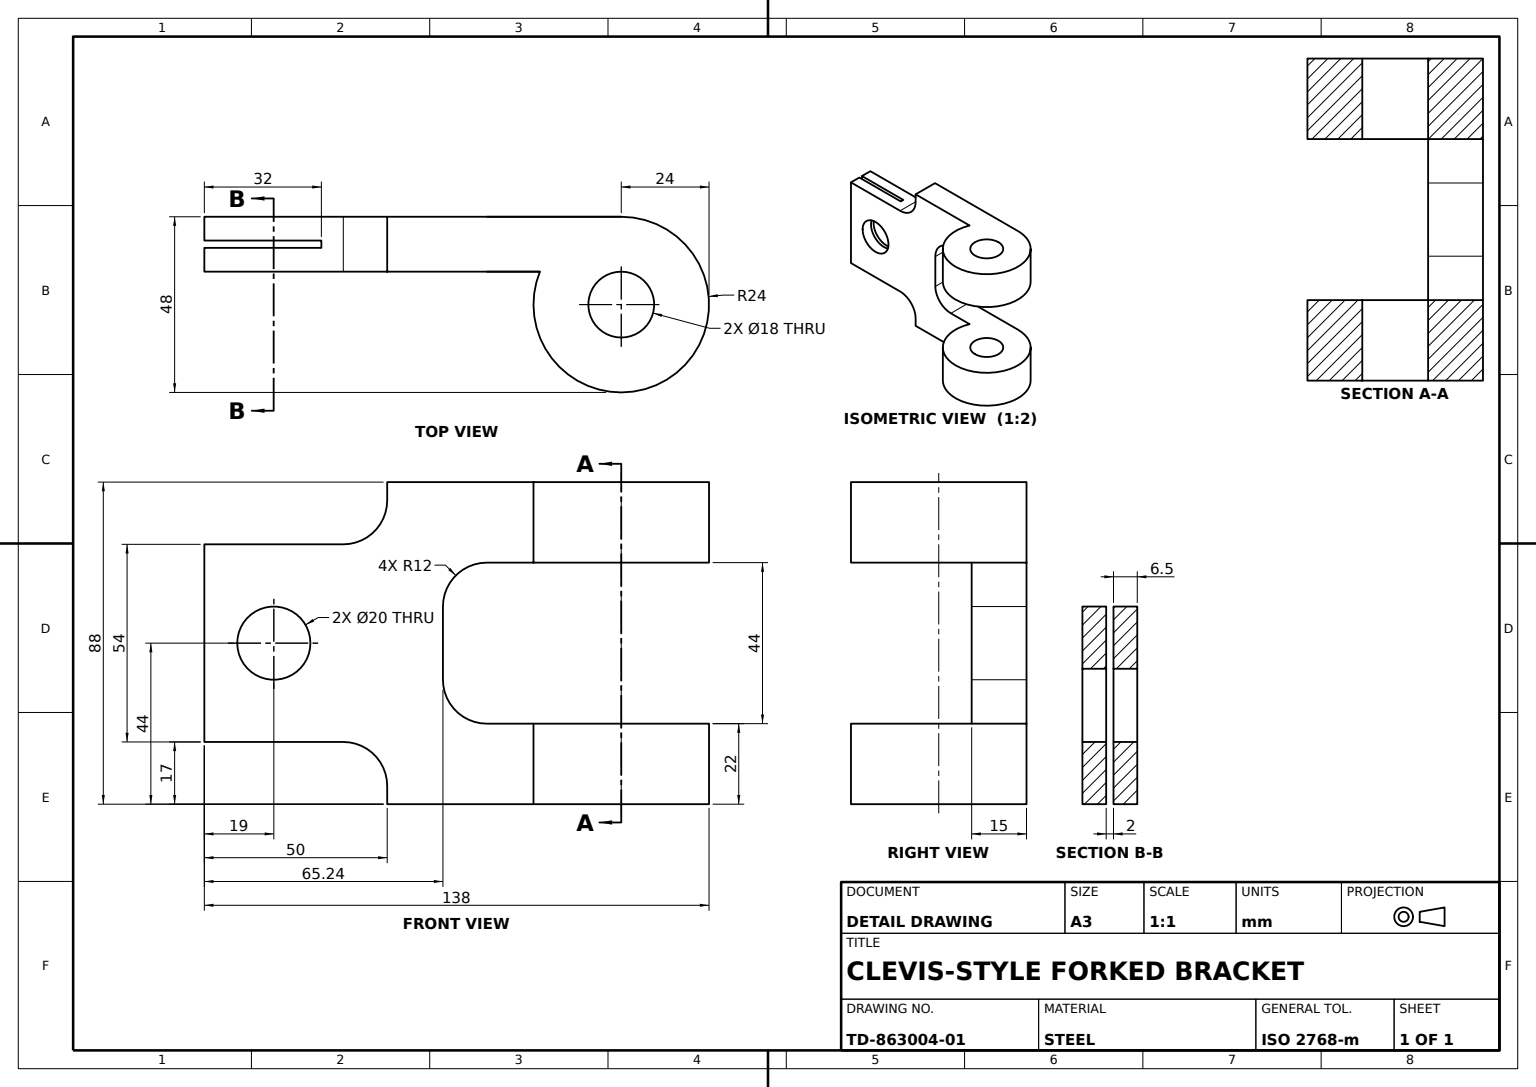
SolidWorks part; units mm, degrees
material "Plain Carbon Steel"
ref_plane "Front Plane" through (0, 0, 0) normal (0, 0, 1) x (1, 0, 0)
ref_plane "Top Plane" through (0, 0, 0) normal (0, 1, 0) x (1, 0, 0)
ref_plane "Right Plane" through (0, 0, 0) normal (1, 0, 0) x (0, 0, -1)
sketch "Base Plate Profile" plane through (0, 0, 0) normal (0, 0, 1) x (1, 0, 0)
  line L0 (0, 0) -> (64, 0)
  line L1 (0, 0) -> (0, -88)
  line L2 (0, -88) -> (64, -88)
  line L3 (64, -88) -> (64, -66)
  line L4 (64, -66) -> (27.24, -66)
  line L5 (15.24, -54) -> (15.24, -34)
  line L6 (27.24, -22) -> (64, -22)
  line L7 (64, -22) -> (64, 0)
  arc A0 (15.24, -54) -> (27.24, -66) centre (27.24, -54) ccw
  arc A1 (27.24, -22) -> (15.24, -34) centre (27.24, -34) ccw
  dimension "D1" = 12
  dimension "D3" = 12
  dimension "D2" = 22
  dimension "D4" = 44
  dimension "D5" = 64
  dimension "D6" = 88
  dimension "D7" = 66
  dimension "D8" = 36.76
extrude "Base Plate" add sketch "Base Plate Profile" along normal blind 15
sketch "Pivot Boss 1 Profile" plane through (0, 0, 0) normal (0, 1, 0) x (1, 0, 0)
  line L0 (0, -15) -> (0, 0) construction
  line L1 (64, 0) -> (0, 0) construction
  circle A0 centre (64, -24) radius 24
  dimension "D1" = 48
  dimension "D2" = 64
  dimension "D3" = 24
extrude "Pivot Boss 1" add sketch "Pivot Boss 1 Profile" against normal blind 22
sketch "Pivot Boss 2 Profile" plane through (0, -88, 0) normal (0, -1, 0) x (1, 0, 0)
  circle A0 centre (64, 24) radius 24
  dimension "D1" = 48
extrude "Pivot Boss 2" add sketch "Pivot Boss 2 Profile" against normal blind 22
sketch "Upright Web Profile" plane through (0, 0, 0) normal (0, 0, -1) x (-1, 0, 0)
  line L0 (0, -44) -> (0, -17)
  line L1 (0, 0) -> (0, -88) construction
  line L2 (0, -44) -> (0, -71)
  line L3 (12, -71) -> (50, -71)
  line L4 (50, -71) -> (50, -17)
  line L5 (50, -17) -> (12, -17)
  line L6 (0, -83) -> (0, -71)
  line L7 (0, -5) -> (0, -17)
  line L8 (-64, 0) -> (0, 0) construction
  arc A0 (0, -5) -> (12, -17) centre (12, -5) ccw
  arc A1 (12, -71) -> (0, -83) centre (12, -83) ccw
  dimension "D1" = 12
  dimension "D2" = 50
  dimension "D3" = 17
extrude "Upright Web" add sketch "Upright Web Profile" against normal blind 15
sketch "Web Slot Profile" plane through (0, -17, 0) normal (0, 1, 0) x (1, 0, 0)
  line L0 (-50, -7.5) -> (-50, -6.5)
  line L1 (-50, -15) -> (-50, 0) construction
  line L2 (-50, -6.5) -> (-18, -6.5)
  line L3 (-18, -6.5) -> (-18, -8.5)
  line L4 (-18, -8.5) -> (-50, -8.5)
  line L5 (-50, -8.5) -> (-50, -7.5)
  line L6 (-50, 0) -> (-12, 0) construction
  dimension "D1" = 32
  dimension "D2" = 6.5
extrude "Web Slot" cut sketch "Web Slot Profile" against normal blind 55
sketch "Web Hole Profile" plane through (0, 0, 15) normal (0, 0, 1) x (1, 0, 0)
  line L0 (41.7514, 0) -> (41.7514, -22) construction
  line L1 (41.7514, 0) -> (0, 0) construction
  circle A0 centre (-31, -44) radius 10
  dimension "D1" = 20
  dimension "D2" = 72.7514
  dimension "D3" = 44
extrude "Web Hole" cut sketch "Web Hole Profile" against normal blind 55
sketch "Pivot Bore Profile" plane through (0, 0, 0) normal (0, 1, 0) x (1, 0, 0)
  circle A0 centre (64, -24) radius 9
  dimension "D1" = 18
extrude "Pivot Bore Through" cut sketch "Pivot Bore Profile" against normal blind 90
